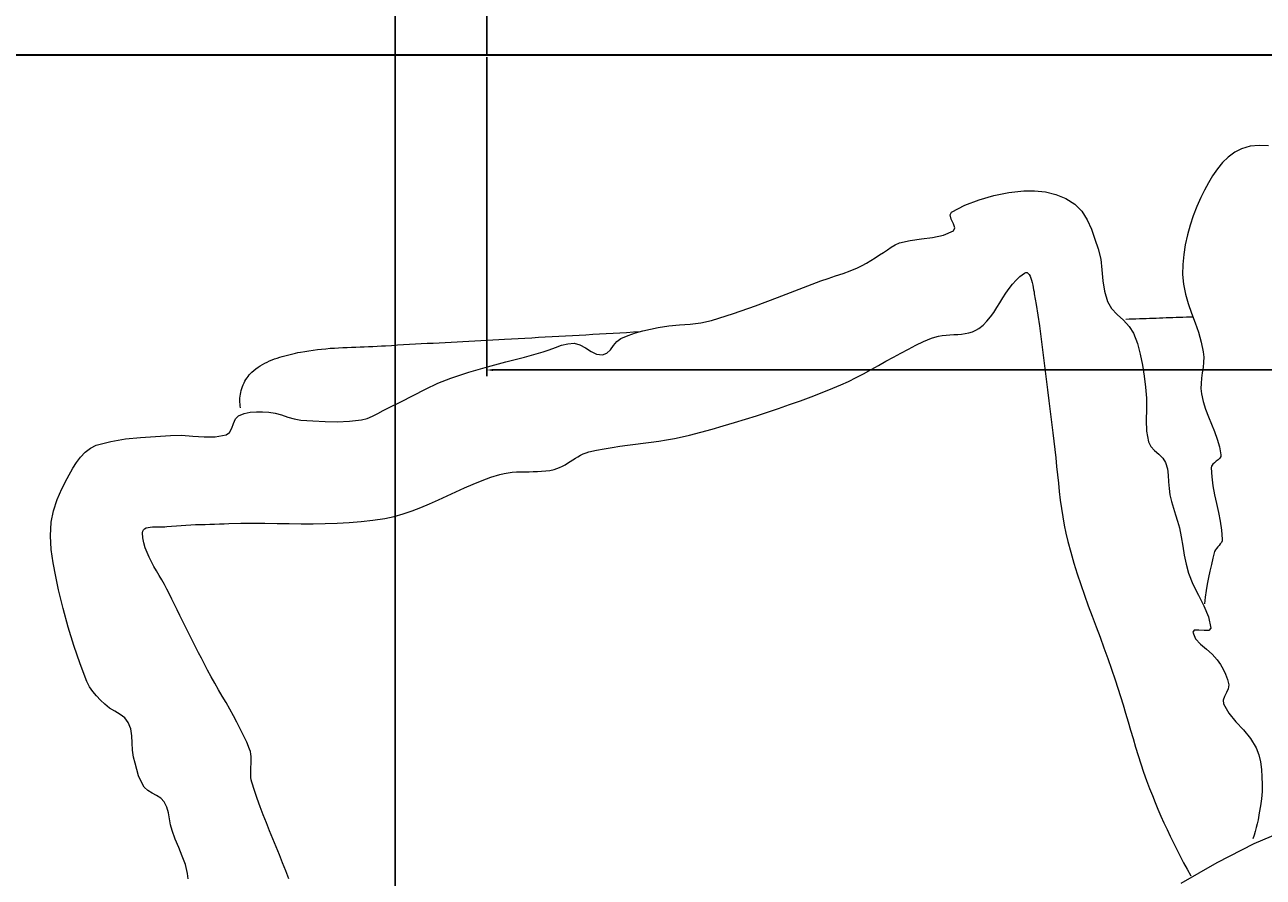
# Model space of a CAD drawing. Units: inches. Extents: x 1770 to 2988, y 1161 to 3221.
# Tile 16 of 44: x 2194 to 2229, y 2344 to 2369. Entities that reach past the tile are written whole.
import ezdxf

# ---------------------------------------------------------------- set-up
doc = ezdxf.new("R2010")
doc.units = ezdxf.units.IN
for name, color, linetype, lineweight in [('A-ANNO-DIMS', 2, 'Continuous', 18), ('A-FURN', 8, 'Continuous', 13), ('A-GLAZ', 4, 'Continuous', 18), ('A-WALL', 7, 'Continuous', 35)]:
    doc.layers.add(name, color=color, linetype=linetype, lineweight=lineweight)
doc.styles.get("Standard").update_dxf_attribs({"font": 'arial.ttf'})
doc.dimstyles.get("Standard").update_dxf_attribs({"dimtxt": 0.18, "dimasz": 0.18, "dimexe": 0.18, "dimexo": 0.0625, "dimgap": 0.09, "dimtad": 0, "dimtih": 1, "dimtoh": 1, "dimdec": 4, "dimzin": 0, "dimdsep": 46, "dimtxsty": 'Standard', "dimcen": 0.09, "dimadec": 0, "dimazin": 0, "dimtfac": 1, "dimtdec": 4, "dimtofl": 0, "dimtmove": 0, "dimatfit": 3, "dimfxl": 1, "dimtolj": 1, "dimtzin": 0, "dimarcsym": 0})

# ---------------------------------------------------------------- blocks, each defined once
blk = doc.blocks.new('BED-DOUBLE-PLAN')
for p, q in [((35.385, 105.421), (35.203, 105.287)), ((35.584, 105.525), (35.385, 105.421)), ((35.831, 105.596), (35.584, 105.525)), ((36.086, 105.618), (35.831, 105.596)), ((36.348, 105.604), (36.086, 105.618)), ((35.039, 105.128), (34.89, 104.949)), ((35.203, 105.287), (35.039, 105.128)), ((34.755, 104.754), (34.633, 104.551)), ((34.89, 104.949), (34.755, 104.754)), ((34.633, 104.551), (34.523, 104.343)), ((27.681, 103.909), (28.087, 104.068)), ((28.087, 104.068), (28.506, 104.19)), ((28.506, 104.19), (28.933, 104.274)), ((28.933, 104.274), (29.364, 104.322)), ((29.364, 104.322), (29.669, 104.325)), ((29.669, 104.325), (29.977, 104.292)), ((29.977, 104.292), (30.279, 104.22)), ((30.279, 104.22), (30.562, 104.105)), ((30.562, 104.105), (30.817, 103.944)), ((34.422, 104.135), (34.307, 103.876)), ((34.523, 104.343), (34.422, 104.135)), ((27.256, 103.634), (27.295, 103.714)), ((27.295, 103.714), (27.681, 103.909)), ((30.817, 103.944), (31.018, 103.741)), ((31.018, 103.741), (31.173, 103.496)), ((34.307, 103.876), (34.203, 103.61)), ((27.291, 103.514), (27.256, 103.634)), ((27.352, 103.382), (27.291, 103.514)), ((27.388, 103.262), (27.352, 103.382)), ((31.173, 103.496), (31.294, 103.225)), ((34.112, 103.338), (34.035, 103.063)), ((34.203, 103.61), (34.112, 103.338)), ((26.119, 102.906), (26.438, 102.948)), ((26.438, 102.948), (26.756, 102.988)), ((26.756, 102.988), (27.064, 103.056)), ((27.064, 103.056), (27.349, 103.179)), ((27.349, 103.179), (27.388, 103.262)), ((31.294, 103.225), (31.395, 102.942)), ((31.395, 102.942), (31.487, 102.661)), ((34.035, 103.063), (33.974, 102.783)), ((25.354, 102.561), (25.464, 102.639)), ((25.464, 102.639), (25.574, 102.714)), ((25.574, 102.714), (25.689, 102.781)), ((25.689, 102.781), (25.811, 102.832)), ((25.811, 102.832), (26.119, 102.906)), ((31.487, 102.661), (31.558, 102.366)), ((33.974, 102.783), (33.93, 102.502)), ((24.742, 102.187), (24.869, 102.258)), ((24.869, 102.258), (24.993, 102.335)), ((24.993, 102.335), (25.117, 102.412)), ((25.117, 102.412), (25.242, 102.489)), ((25.242, 102.489), (25.354, 102.561)), ((31.558, 102.366), (31.593, 102.061)), ((33.93, 102.502), (33.904, 102.219)), ((23.778, 101.819), (23.988, 101.89)), ((23.988, 101.89), (24.198, 101.962)), ((24.198, 101.962), (24.406, 102.038)), ((24.406, 102.038), (24.611, 102.123)), ((24.611, 102.123), (24.742, 102.187)), ((29.139, 101.774), (29.253, 101.879)), ((29.253, 101.879), (29.38, 101.971)), ((29.38, 101.971), (29.42, 101.987)), ((29.42, 101.987), (29.457, 101.984)), ((29.457, 101.984), (29.489, 101.964)), ((29.489, 101.964), (29.518, 101.93)), ((29.518, 101.93), (29.543, 101.885)), ((29.543, 101.885), (29.566, 101.829)), ((31.593, 102.061), (31.62, 101.753)), ((33.904, 102.219), (33.898, 101.936)), ((33.898, 101.936), (33.922, 101.653)), ((22.945, 101.514), (23.568, 101.747)), ((23.568, 101.747), (23.778, 101.819)), ((28.85, 101.399), (28.939, 101.531)), ((28.939, 101.531), (29.035, 101.657)), ((29.035, 101.657), (29.139, 101.774)), ((29.566, 101.829), (29.586, 101.767)), ((29.586, 101.767), (29.603, 101.7)), ((29.603, 101.7), (29.618, 101.631)), ((29.618, 101.631), (29.631, 101.561)), ((29.631, 101.561), (29.643, 101.495)), ((31.62, 101.753), (31.664, 101.452)), ((33.922, 101.653), (33.978, 101.374)), ((21.701, 101.039), (22.324, 101.275)), ((22.324, 101.275), (22.945, 101.514)), ((28.679, 101.123), (28.763, 101.262)), ((28.763, 101.262), (28.85, 101.399)), ((29.643, 101.495), (29.653, 101.433)), ((29.653, 101.433), (29.662, 101.379)), ((29.662, 101.379), (29.714, 101.076)), ((31.664, 101.452), (31.751, 101.162)), ((33.978, 101.374), (34.058, 101.099)), ((20.44, 100.618), (21.074, 100.817)), ((21.074, 100.817), (21.701, 101.039)), ((28.411, 100.721), (28.505, 100.85)), ((28.505, 100.85), (28.593, 100.985)), ((28.593, 100.985), (28.679, 101.123)), ((29.714, 101.076), (29.763, 100.772)), ((31.751, 101.162), (31.871, 100.963)), ((31.871, 100.963), (32.032, 100.788)), ((34.058, 101.099), (34.153, 100.826)), ((34.153, 100.826), (34.252, 100.553)), ((18.918, 100.416), (19.222, 100.462)), ((19.222, 100.462), (19.529, 100.49)), ((19.529, 100.49), (19.836, 100.515)), ((19.836, 100.515), (20.141, 100.553)), ((20.141, 100.553), (20.44, 100.618)), ((28.077, 100.392), (28.2, 100.489)), ((28.2, 100.489), (28.31, 100.6)), ((28.31, 100.6), (28.411, 100.721)), ((29.763, 100.772), (29.808, 100.467)), ((29.808, 100.467), (29.85, 100.162)), ((32.032, 100.788), (32.208, 100.623)), ((32.208, 100.623), (32.371, 100.449)), ((32.279, 100.659), (32.375, 100.663)), ((32.375, 100.663), (32.47, 100.666)), ((32.47, 100.666), (32.566, 100.669)), ((32.566, 100.669), (32.662, 100.673)), ((32.662, 100.673), (32.758, 100.676)), ((32.758, 100.676), (32.854, 100.679)), ((32.854, 100.679), (32.949, 100.683)), ((32.949, 100.683), (33.045, 100.686)), ((33.045, 100.686), (33.141, 100.689)), ((33.141, 100.689), (33.237, 100.693)), ((33.237, 100.693), (33.333, 100.696)), ((33.333, 100.696), (33.429, 100.7)), ((33.429, 100.7), (33.524, 100.703)), ((33.524, 100.703), (33.62, 100.706)), ((33.62, 100.706), (33.716, 100.71)), ((33.716, 100.71), (33.812, 100.713)), ((33.812, 100.713), (33.908, 100.716)), ((33.908, 100.716), (34.004, 100.72)), ((34.004, 100.72), (34.099, 100.723)), ((34.099, 100.723), (34.195, 100.726)), ((34.252, 100.553), (34.347, 100.28)), ((14.92, 100.104), (15.114, 100.115)), ((15.114, 100.115), (15.308, 100.126)), ((15.308, 100.126), (15.501, 100.137)), ((15.501, 100.137), (15.695, 100.147)), ((15.695, 100.147), (15.888, 100.158)), ((15.888, 100.158), (16.082, 100.169)), ((16.082, 100.169), (16.276, 100.18)), ((16.276, 100.18), (16.469, 100.191)), ((16.469, 100.191), (16.663, 100.202)), ((16.663, 100.202), (16.857, 100.213)), ((16.857, 100.213), (17.05, 100.224)), ((17.05, 100.224), (17.244, 100.235)), ((17.244, 100.235), (17.437, 100.246)), ((17.437, 100.246), (17.631, 100.257)), ((17.631, 100.257), (17.825, 100.268)), ((17.825, 100.268), (18.018, 100.279)), ((17.853, 100.102), (18.057, 100.19)), ((18.018, 100.279), (18.212, 100.29)), ((18.057, 100.19), (18.267, 100.262)), ((18.212, 100.29), (18.406, 100.301)), ((18.267, 100.262), (18.482, 100.321)), ((18.482, 100.321), (18.7, 100.371)), ((18.7, 100.371), (18.918, 100.416)), ((26.5, 100.015), (26.723, 100.111)), ((26.723, 100.111), (26.823, 100.146)), ((26.823, 100.146), (26.927, 100.171)), ((26.927, 100.171), (27.034, 100.188)), ((27.034, 100.188), (27.143, 100.2)), ((27.143, 100.2), (27.253, 100.208)), ((27.253, 100.208), (27.363, 100.215)), ((27.363, 100.215), (27.473, 100.222)), ((27.473, 100.222), (27.582, 100.232)), ((27.582, 100.232), (27.688, 100.246)), ((27.688, 100.246), (27.792, 100.267)), ((27.792, 100.267), (27.892, 100.297)), ((27.892, 100.297), (27.987, 100.338)), ((27.987, 100.338), (28.077, 100.392)), ((29.85, 100.162), (29.89, 99.857)), ((32.371, 100.449), (32.495, 100.252)), ((32.495, 100.252), (32.606, 99.957)), ((34.347, 100.28), (34.429, 100.003)), ((8.824, 99.736), (8.944, 99.756)), ((8.944, 99.756), (9.065, 99.773)), ((9.065, 99.773), (9.185, 99.788)), ((9.185, 99.788), (9.306, 99.802)), ((9.306, 99.802), (9.428, 99.813)), ((9.428, 99.813), (9.549, 99.823)), ((9.549, 99.823), (9.671, 99.831)), ((9.671, 99.831), (9.792, 99.839)), ((9.792, 99.839), (9.914, 99.845)), ((9.914, 99.845), (10.036, 99.851)), ((10.036, 99.851), (10.158, 99.855)), ((10.158, 99.855), (10.28, 99.86)), ((10.28, 99.86), (10.403, 99.864)), ((10.403, 99.864), (10.525, 99.869)), ((10.525, 99.869), (10.647, 99.873)), ((10.647, 99.873), (10.769, 99.878)), ((10.769, 99.878), (10.891, 99.883)), ((10.891, 99.883), (11.012, 99.89)), ((11.012, 99.89), (11.134, 99.897)), ((11.134, 99.897), (11.304, 99.907)), ((11.304, 99.907), (11.474, 99.918)), ((11.474, 99.918), (11.644, 99.928)), ((11.644, 99.928), (11.814, 99.938)), ((11.814, 99.938), (11.984, 99.947)), ((11.984, 99.947), (12.154, 99.957)), ((12.154, 99.957), (12.324, 99.966)), ((12.324, 99.966), (12.493, 99.975)), ((12.493, 99.975), (12.663, 99.984)), ((12.663, 99.984), (12.833, 99.993)), ((12.833, 99.993), (13.003, 100.002)), ((13.003, 100.002), (13.173, 100.011)), ((13.173, 100.011), (13.343, 100.019)), ((13.343, 100.019), (13.513, 100.028)), ((13.513, 100.028), (13.683, 100.037)), ((13.683, 100.037), (13.853, 100.046)), ((13.853, 100.046), (14.023, 100.055)), ((14.023, 100.055), (14.193, 100.064)), ((14.193, 100.064), (14.363, 100.073)), ((14.363, 100.073), (14.533, 100.083)), ((14.533, 100.083), (14.727, 100.093)), ((14.727, 100.093), (14.92, 100.104)), ((15.635, 99.718), (15.81, 99.777)), ((15.81, 99.777), (15.984, 99.845)), ((15.984, 99.845), (16.159, 99.909)), ((16.159, 99.909), (16.336, 99.954)), ((16.336, 99.954), (16.516, 99.966)), ((16.516, 99.966), (16.685, 99.923)), ((16.685, 99.923), (16.844, 99.835)), ((16.844, 99.835), (17.001, 99.735)), ((17.452, 99.683), (17.553, 99.78)), ((17.553, 99.78), (17.645, 99.9)), ((17.645, 99.9), (17.741, 100.016)), ((17.741, 100.016), (17.853, 100.102)), ((25.85, 99.689), (26.064, 99.803)), ((26.064, 99.803), (26.281, 99.912)), ((26.281, 99.912), (26.5, 100.015)), ((29.89, 99.857), (29.929, 99.551)), ((32.606, 99.957), (32.689, 99.653)), ((34.429, 100.003), (34.488, 99.723)), ((7.619, 99.363), (7.685, 99.399)), ((7.685, 99.399), (7.753, 99.432)), ((7.753, 99.432), (7.822, 99.463)), ((7.822, 99.463), (7.892, 99.493)), ((7.892, 99.493), (7.964, 99.52)), ((7.964, 99.52), (8.036, 99.546)), ((8.036, 99.546), (8.109, 99.569)), ((8.109, 99.569), (8.183, 99.591)), ((8.183, 99.591), (8.258, 99.612)), ((8.258, 99.612), (8.332, 99.632)), ((8.332, 99.632), (8.407, 99.65)), ((8.407, 99.65), (8.482, 99.667)), ((8.482, 99.667), (8.556, 99.684)), ((8.556, 99.684), (8.631, 99.699)), ((8.631, 99.699), (8.705, 99.714)), ((8.705, 99.714), (8.824, 99.736)), ((14.041, 99.297), (14.572, 99.437)), ((14.572, 99.437), (15.105, 99.574)), ((15.105, 99.574), (15.635, 99.718)), ((17.001, 99.735), (17.16, 99.657)), ((17.16, 99.657), (17.329, 99.635)), ((17.329, 99.635), (17.452, 99.683)), ((25.212, 99.334), (25.424, 99.453)), ((25.424, 99.453), (25.636, 99.572)), ((25.636, 99.572), (25.85, 99.689)), ((29.929, 99.551), (29.966, 99.246)), ((32.689, 99.653), (32.75, 99.342)), ((34.496, 99.425), (34.48, 99.274)), ((34.488, 99.723), (34.501, 99.574)), ((34.501, 99.574), (34.496, 99.425)), ((7.207, 99.023), (7.241, 99.066)), ((7.241, 99.066), (7.278, 99.106)), ((7.278, 99.106), (7.316, 99.144)), ((7.316, 99.144), (7.372, 99.193)), ((7.372, 99.193), (7.431, 99.24)), ((7.431, 99.24), (7.491, 99.283)), ((7.491, 99.283), (7.554, 99.324)), ((7.554, 99.324), (7.619, 99.363)), ((12.992, 98.973), (13.513, 99.145)), ((13.513, 99.145), (14.041, 99.297)), ((24.571, 98.986), (24.786, 99.099)), ((24.786, 99.099), (25, 99.215)), ((25, 99.215), (25.212, 99.334)), ((29.966, 99.246), (30.003, 98.94)), ((32.75, 99.342), (32.799, 99.027)), ((34.459, 99.124), (34.438, 98.973)), ((34.48, 99.274), (34.459, 99.124)), ((7.028, 98.674), (7.046, 98.728)), ((7.046, 98.728), (7.067, 98.781)), ((7.067, 98.781), (7.091, 98.833)), ((7.091, 98.833), (7.117, 98.883)), ((7.117, 98.883), (7.144, 98.931)), ((7.144, 98.931), (7.175, 98.978)), ((7.175, 98.978), (7.207, 99.023)), ((12.273, 98.658), (12.628, 98.826)), ((12.628, 98.826), (12.992, 98.973)), ((23.911, 98.681), (24.134, 98.776)), ((24.134, 98.776), (24.354, 98.878)), ((24.354, 98.878), (24.571, 98.986)), ((30.003, 98.94), (30.039, 98.634)), ((32.799, 99.027), (32.842, 98.713)), ((32.842, 98.713), (32.864, 98.4)), ((34.423, 98.823), (34.42, 98.674)), ((34.438, 98.973), (34.423, 98.823)), ((6.971, 98.342), (6.974, 98.397)), ((6.971, 98.287), (6.971, 98.342)), ((6.974, 98.397), (6.979, 98.453)), ((6.979, 98.453), (6.987, 98.509)), ((6.987, 98.509), (6.998, 98.565)), ((6.998, 98.565), (7.012, 98.62)), ((7.012, 98.62), (7.028, 98.674)), ((11.572, 98.299), (11.922, 98.48)), ((11.922, 98.48), (12.273, 98.658)), ((22.983, 98.327), (23.293, 98.442)), ((23.293, 98.442), (23.603, 98.56)), ((23.603, 98.56), (23.911, 98.681)), ((30.039, 98.634), (30.076, 98.328)), ((32.864, 98.4), (32.862, 98.084)), ((34.42, 98.674), (34.435, 98.525)), ((34.435, 98.525), (34.485, 98.303)), ((6.975, 98.232), (6.971, 98.287)), ((6.981, 98.178), (6.975, 98.232)), ((6.99, 98.125), (6.981, 98.178)), ((7.094, 97.962), (7.265, 97.998)), ((7.265, 97.998), (7.442, 98.012)), ((7.442, 98.012), (7.621, 98.01)), ((7.621, 98.01), (7.798, 98)), ((7.798, 98), (7.983, 97.971)), ((10.916, 97.961), (11.066, 98.046)), ((11.066, 98.046), (11.219, 98.125)), ((11.219, 98.125), (11.572, 98.299)), ((21.728, 97.898), (22.043, 98)), ((22.043, 98), (22.358, 98.106)), ((22.358, 98.106), (22.671, 98.215)), ((22.671, 98.215), (22.983, 98.327)), ((30.076, 98.328), (30.113, 98.022)), ((30.113, 98.022), (30.152, 97.716)), ((32.862, 98.084), (32.856, 97.768)), ((34.485, 98.303), (34.554, 98.085)), ((34.554, 98.085), (34.635, 97.87)), ((6.737, 97.54), (6.785, 97.678)), ((6.785, 97.678), (6.843, 97.807)), ((6.843, 97.807), (6.934, 97.897)), ((6.934, 97.897), (7.094, 97.962)), ((7.983, 97.971), (8.164, 97.919)), ((8.164, 97.919), (8.344, 97.86)), ((8.344, 97.86), (8.526, 97.807)), ((8.526, 97.807), (8.711, 97.775)), ((8.711, 97.775), (9.057, 97.749)), ((9.057, 97.749), (9.404, 97.731)), ((9.404, 97.731), (9.752, 97.727)), ((9.752, 97.727), (10.099, 97.741)), ((10.099, 97.741), (10.443, 97.776)), ((10.443, 97.776), (10.607, 97.816)), ((10.607, 97.816), (10.764, 97.881)), ((10.764, 97.881), (10.916, 97.961)), ((20.777, 97.608), (21.095, 97.702)), ((21.095, 97.702), (21.412, 97.798)), ((21.412, 97.798), (21.728, 97.898)), ((30.152, 97.716), (30.192, 97.411)), ((32.856, 97.768), (32.868, 97.455)), ((34.635, 97.87), (34.722, 97.657)), ((34.722, 97.657), (34.808, 97.443)), ((3.703, 97.235), (4.13, 97.276)), ((4.13, 97.276), (4.56, 97.305)), ((4.56, 97.305), (4.988, 97.334)), ((4.988, 97.334), (5.307, 97.338)), ((5.307, 97.338), (5.628, 97.316)), ((5.628, 97.316), (5.949, 97.294)), ((5.949, 97.294), (6.266, 97.297)), ((6.266, 97.297), (6.576, 97.352)), ((6.576, 97.352), (6.675, 97.422)), ((6.675, 97.422), (6.737, 97.54)), ((19.381, 97.247), (19.6, 97.292)), ((19.6, 97.292), (19.818, 97.344)), ((19.818, 97.344), (20.138, 97.429)), ((20.138, 97.429), (20.458, 97.517)), ((20.458, 97.517), (20.777, 97.608)), ((30.192, 97.411), (30.222, 97.172)), ((32.868, 97.455), (32.921, 97.148)), ((34.808, 97.443), (34.886, 97.228)), ((2.554, 96.859), (2.703, 96.975)), ((2.703, 96.975), (2.87, 97.055)), ((2.87, 97.055), (3.281, 97.166)), ((3.281, 97.166), (3.703, 97.235)), ((17.161, 96.913), (17.38, 96.957)), ((17.38, 96.957), (17.602, 96.995)), ((17.602, 96.995), (17.824, 97.028)), ((17.824, 97.028), (18.046, 97.058)), ((18.046, 97.058), (18.269, 97.086)), ((18.269, 97.086), (18.493, 97.114)), ((18.493, 97.114), (18.716, 97.143)), ((18.716, 97.143), (18.938, 97.174)), ((18.938, 97.174), (19.16, 97.208)), ((19.16, 97.208), (19.381, 97.247)), ((30.222, 97.172), (30.25, 96.932)), ((30.25, 96.932), (30.275, 96.692)), ((32.921, 97.148), (32.988, 97.015)), ((32.988, 97.015), (33.094, 96.903)), ((34.886, 97.228), (34.95, 97.009)), ((34.95, 97.009), (34.993, 96.785)), ((2.307, 96.562), (2.422, 96.718)), ((2.422, 96.718), (2.554, 96.859)), ((16.332, 96.542), (16.406, 96.589)), ((16.406, 96.589), (16.48, 96.636)), ((16.48, 96.636), (16.554, 96.682)), ((16.554, 96.682), (16.628, 96.726)), ((16.628, 96.726), (16.704, 96.768)), ((16.704, 96.768), (16.781, 96.805)), ((16.781, 96.805), (16.86, 96.837)), ((16.86, 96.837), (16.942, 96.862)), ((16.942, 96.862), (17.161, 96.913)), ((30.275, 96.692), (30.3, 96.452)), ((33.094, 96.903), (33.215, 96.799)), ((33.215, 96.799), (33.328, 96.689)), ((33.328, 96.689), (33.41, 96.561)), ((34.86, 96.597), (34.806, 96.555)), ((34.912, 96.639), (34.86, 96.597)), ((34.957, 96.683), (34.912, 96.639)), ((34.986, 96.731), (34.957, 96.683)), ((34.993, 96.785), (34.986, 96.731)), ((2.039, 96.109), (2.205, 96.4)), ((2.205, 96.4), (2.307, 96.562)), ((14.142, 96.14), (14.4, 96.222)), ((14.4, 96.222), (14.516, 96.251)), ((14.516, 96.251), (14.632, 96.271)), ((14.632, 96.271), (14.751, 96.284)), ((14.751, 96.284), (14.87, 96.293)), ((14.87, 96.293), (14.99, 96.297)), ((14.99, 96.297), (15.11, 96.299)), ((15.11, 96.299), (15.23, 96.299)), ((15.23, 96.299), (15.351, 96.301)), ((15.351, 96.301), (15.471, 96.304)), ((15.471, 96.304), (15.591, 96.31)), ((15.591, 96.31), (15.71, 96.321)), ((15.71, 96.321), (15.827, 96.338)), ((15.827, 96.338), (15.944, 96.363)), ((15.944, 96.363), (16.026, 96.388)), ((16.026, 96.388), (16.105, 96.419)), ((16.105, 96.419), (16.182, 96.456)), ((16.182, 96.456), (16.258, 96.498)), ((16.258, 96.498), (16.332, 96.542)), ((30.3, 96.452), (30.324, 96.211)), ((33.41, 96.561), (33.462, 96.384)), ((33.462, 96.384), (33.486, 96.199)), ((34.725, 96.462), (34.713, 96.407)), ((34.713, 96.407), (34.729, 96.151)), ((34.759, 96.511), (34.725, 96.462)), ((34.806, 96.555), (34.759, 96.511)), ((1.884, 95.809), (2.039, 96.109)), ((13.385, 95.836), (13.635, 95.945)), ((13.635, 95.945), (13.887, 96.047)), ((13.887, 96.047), (14.142, 96.14)), ((30.324, 96.211), (30.349, 95.971)), ((30.349, 95.971), (30.375, 95.731)), ((33.486, 96.199), (33.497, 96.01)), ((33.497, 96.01), (33.509, 95.822)), ((34.729, 96.151), (34.763, 95.896)), ((34.763, 95.896), (34.811, 95.643)), ((1.749, 95.501), (1.884, 95.809)), ((12.641, 95.494), (12.889, 95.608)), ((12.889, 95.608), (13.137, 95.723)), ((13.137, 95.723), (13.385, 95.836)), ((30.375, 95.731), (30.404, 95.491)), ((33.509, 95.822), (33.535, 95.636)), ((33.535, 95.636), (33.582, 95.446)), ((34.811, 95.643), (34.865, 95.39)), ((1.583, 94.858), (1.646, 95.184)), ((1.646, 95.184), (1.749, 95.501)), ((11.633, 95.096), (11.889, 95.182)), ((11.889, 95.182), (12.142, 95.279)), ((12.142, 95.279), (12.392, 95.383)), ((12.392, 95.383), (12.641, 95.494)), ((30.404, 95.491), (30.436, 95.252)), ((30.436, 95.252), (30.473, 95.014)), ((33.582, 95.446), (33.638, 95.258)), ((33.638, 95.258), (33.698, 95.071)), ((34.865, 95.39), (34.921, 95.137)), ((1.562, 94.471), (1.583, 94.858)), ((5.976, 94.796), (6.112, 94.8)), ((6.112, 94.8), (6.249, 94.804)), ((6.249, 94.804), (6.385, 94.808)), ((6.385, 94.808), (6.522, 94.812)), ((6.522, 94.812), (6.658, 94.817)), ((6.658, 94.817), (7.001, 94.826)), ((7.001, 94.826), (7.344, 94.829)), ((7.344, 94.829), (7.688, 94.827)), ((7.688, 94.827), (8.032, 94.823)), ((8.032, 94.823), (8.376, 94.818)), ((8.376, 94.818), (8.721, 94.814)), ((8.721, 94.814), (9.064, 94.813)), ((9.064, 94.813), (9.408, 94.816)), ((9.408, 94.816), (9.75, 94.826)), ((9.75, 94.826), (10.092, 94.844)), ((10.092, 94.844), (10.433, 94.873)), ((10.433, 94.873), (10.772, 94.913)), ((10.772, 94.913), (11.11, 94.966)), ((11.11, 94.966), (11.374, 95.023)), ((11.374, 95.023), (11.633, 95.096)), ((30.473, 95.014), (30.515, 94.777)), ((33.698, 95.071), (33.755, 94.883)), ((33.755, 94.883), (33.806, 94.694)), ((34.921, 95.137), (34.971, 94.884)), ((34.971, 94.884), (35.009, 94.629)), ((1.584, 94.082), (1.562, 94.471)), ((4.189, 94.55), (4.196, 94.6)), ((4.202, 94.406), (4.189, 94.55)), ((4.196, 94.6), (4.217, 94.64)), ((4.217, 94.64), (4.251, 94.67)), ((4.251, 94.67), (4.296, 94.693)), ((4.296, 94.693), (4.35, 94.708)), ((4.35, 94.708), (4.412, 94.718)), ((4.412, 94.718), (4.479, 94.724)), ((4.479, 94.724), (4.55, 94.727)), ((4.55, 94.727), (4.622, 94.727)), ((4.622, 94.727), (4.693, 94.727)), ((4.693, 94.727), (4.762, 94.727)), ((4.762, 94.727), (4.827, 94.728)), ((4.827, 94.728), (4.886, 94.732)), ((4.886, 94.732), (5.022, 94.746)), ((5.022, 94.746), (5.158, 94.757)), ((5.158, 94.757), (5.294, 94.767)), ((5.294, 94.767), (5.43, 94.775)), ((5.43, 94.775), (5.566, 94.782)), ((5.566, 94.782), (5.703, 94.787)), ((5.703, 94.787), (5.839, 94.792)), ((5.839, 94.792), (5.976, 94.796)), ((30.515, 94.777), (30.563, 94.541)), ((30.563, 94.541), (30.618, 94.307)), ((33.806, 94.694), (33.859, 94.435)), ((35.009, 94.629), (35.031, 94.373)), ((4.229, 94.265), (4.202, 94.406)), ((4.269, 94.127), (4.229, 94.265)), ((4.319, 93.992), (4.269, 94.127)), ((30.618, 94.307), (30.701, 93.997)), ((33.859, 94.435), (33.903, 94.175)), ((33.903, 94.175), (33.946, 93.914)), ((34.863, 94.11), (34.833, 94.065)), ((34.899, 94.152), (34.863, 94.11)), ((34.938, 94.193), (34.899, 94.152)), ((34.974, 94.235), (34.938, 94.193)), ((35.004, 94.278), (34.974, 94.235)), ((35.024, 94.323), (35.004, 94.278)), ((35.031, 94.373), (35.024, 94.323)), ((1.637, 93.693), (1.584, 94.082)), ((4.378, 93.858), (4.319, 93.992)), ((4.444, 93.726), (4.378, 93.858)), ((30.701, 93.997), (30.791, 93.689)), ((33.946, 93.914), (33.997, 93.655)), ((34.763, 93.833), (34.718, 93.649)), ((34.812, 94.017), (34.763, 93.833)), ((34.833, 94.065), (34.812, 94.017)), ((1.711, 93.307), (1.637, 93.693)), ((4.515, 93.595), (4.444, 93.726)), ((4.59, 93.465), (4.515, 93.595)), ((4.666, 93.336), (4.59, 93.465)), ((30.791, 93.689), (30.887, 93.383)), ((33.997, 93.655), (34.064, 93.401)), ((34.064, 93.401), (34.191, 93.084)), ((34.676, 93.463), (34.637, 93.277)), ((34.718, 93.649), (34.676, 93.463)), ((1.795, 92.924), (1.711, 93.307)), ((4.742, 93.207), (4.666, 93.336)), ((4.817, 93.077), (4.742, 93.207)), ((4.888, 92.947), (4.817, 93.077)), ((30.887, 93.383), (30.989, 93.078)), ((30.989, 93.078), (31.095, 92.775)), ((34.191, 93.084), (34.349, 92.776)), ((34.602, 93.089), (34.571, 92.902)), ((34.637, 93.277), (34.602, 93.089)), ((1.923, 92.391), (1.795, 92.924)), ((4.953, 92.816), (4.888, 92.947)), ((5.027, 92.661), (4.953, 92.816)), ((31.095, 92.775), (31.204, 92.473)), ((34.349, 92.776), (34.507, 92.47)), ((34.543, 92.713), (34.519, 92.525)), ((34.571, 92.902), (34.543, 92.713)), ((2.067, 91.861), (1.923, 92.391)), ((5.102, 92.506), (5.027, 92.661)), ((5.177, 92.351), (5.102, 92.506)), ((5.252, 92.197), (5.177, 92.351)), ((31.204, 92.473), (31.315, 92.172)), ((34.507, 92.47), (34.635, 92.156)), ((5.328, 92.043), (5.252, 92.197)), ((5.405, 91.889), (5.328, 92.043)), ((31.315, 92.172), (31.427, 91.87)), ((34.635, 92.156), (34.701, 91.828)), ((2.227, 91.336), (2.067, 91.861)), ((5.482, 91.736), (5.405, 91.889)), ((5.559, 91.583), (5.482, 91.736)), ((31.427, 91.87), (31.54, 91.569)), ((34.229, 91.774), (34.188, 91.712)), ((34.188, 91.712), (34.269, 91.526)), ((34.357, 91.777), (34.229, 91.774)), ((34.516, 91.761), (34.357, 91.777)), ((34.649, 91.765), (34.516, 91.761)), ((34.701, 91.828), (34.649, 91.765)), ((2.405, 90.816), (2.227, 91.336)), ((5.637, 91.43), (5.559, 91.583)), ((5.715, 91.277), (5.637, 91.43)), ((5.794, 91.124), (5.715, 91.277)), ((31.54, 91.569), (31.652, 91.268)), ((31.652, 91.268), (31.762, 90.966)), ((34.269, 91.526), (34.408, 91.37)), ((34.408, 91.37), (34.576, 91.228)), ((5.872, 90.971), (5.794, 91.124)), ((5.951, 90.819), (5.872, 90.971)), ((31.762, 90.966), (31.869, 90.663)), ((34.576, 91.228), (34.746, 91.085)), ((34.746, 91.085), (34.888, 90.925)), ((34.888, 90.925), (34.975, 90.793)), ((2.601, 90.304), (2.405, 90.816)), ((6.05, 90.63), (5.951, 90.819)), ((6.153, 90.443), (6.05, 90.63)), ((31.869, 90.663), (31.973, 90.359)), ((34.975, 90.793), (35.056, 90.655)), ((35.056, 90.655), (35.126, 90.512)), ((2.675, 90.157), (2.601, 90.304)), ((6.258, 90.258), (6.153, 90.443)), ((6.364, 90.073), (6.258, 90.258)), ((31.973, 90.359), (32.05, 90.12)), ((35.126, 90.512), (35.181, 90.364)), ((35.181, 90.364), (35.215, 90.211)), ((35.215, 90.211), (35.201, 90.1)), ((2.769, 90.021), (2.675, 90.157)), ((2.877, 89.894), (2.769, 90.021)), ((2.994, 89.773), (2.877, 89.894)), ((6.47, 89.888), (6.364, 90.073)), ((6.577, 89.703), (6.47, 89.888)), ((32.05, 90.12), (32.125, 89.88)), ((32.125, 89.88), (32.197, 89.64)), ((35.091, 89.882), (35.052, 89.775)), ((35.151, 89.99), (35.091, 89.882)), ((35.201, 90.1), (35.151, 89.99)), ((3.112, 89.656), (2.994, 89.773)), ((3.247, 89.55), (3.112, 89.656)), ((3.397, 89.459), (3.247, 89.55)), ((6.682, 89.518), (6.577, 89.703)), ((6.786, 89.331), (6.682, 89.518)), ((32.197, 89.64), (32.269, 89.399)), ((35.052, 89.775), (35.063, 89.671)), ((35.063, 89.671), (35.219, 89.402)), ((3.548, 89.369), (3.397, 89.459)), ((3.682, 89.267), (3.548, 89.369)), ((3.785, 89.136), (3.682, 89.267)), ((6.886, 89.144), (6.786, 89.331)), ((6.984, 88.955), (6.886, 89.144)), ((32.269, 89.399), (32.34, 89.158)), ((32.34, 89.158), (32.41, 88.917)), ((35.219, 89.402), (35.418, 89.158)), ((35.418, 89.158), (35.633, 88.923)), ((3.854, 88.952), (3.785, 89.136)), ((3.883, 88.756), (3.854, 88.952)), ((7.077, 88.764), (6.984, 88.955)), ((32.41, 88.917), (32.481, 88.676)), ((35.633, 88.923), (35.836, 88.68)), ((3.892, 88.552), (3.883, 88.756)), ((3.902, 88.348), (3.892, 88.552)), ((7.166, 88.571), (7.077, 88.764)), ((7.248, 88.375), (7.166, 88.571)), ((32.481, 88.676), (32.554, 88.436)), ((32.554, 88.436), (32.628, 88.196)), ((35.836, 88.68), (36.001, 88.415)), ((3.933, 88.15), (3.902, 88.348)), ((3.976, 87.971), (3.933, 88.15)), ((7.271, 88.306), (7.248, 88.375)), ((7.286, 88.236), (7.271, 88.306)), ((7.294, 88.164), (7.286, 88.236)), ((7.296, 88.091), (7.294, 88.164)), ((7.295, 88.017), (7.296, 88.091)), ((32.628, 88.196), (32.705, 87.957)), ((36.001, 88.415), (36.077, 88.217)), ((36.077, 88.217), (36.124, 88.01)), ((4.024, 87.792), (3.976, 87.971)), ((4.08, 87.617), (4.024, 87.792)), ((7.28, 87.718), (7.283, 87.792)), ((7.283, 87.792), (7.287, 87.867)), ((7.287, 87.867), (7.292, 87.942)), ((7.292, 87.942), (7.295, 88.017)), ((32.705, 87.957), (32.785, 87.719)), ((36.124, 88.01), (36.151, 87.797)), ((36.151, 87.797), (36.164, 87.581)), ((4.151, 87.448), (4.08, 87.617)), ((4.242, 87.291), (4.151, 87.448)), ((7.28, 87.644), (7.28, 87.718)), ((7.285, 87.57), (7.28, 87.644)), ((7.295, 87.498), (7.285, 87.57)), ((7.312, 87.428), (7.295, 87.498)), ((7.387, 87.194), (7.312, 87.428)), ((32.785, 87.719), (32.868, 87.483)), ((32.868, 87.483), (32.956, 87.248)), ((36.164, 87.581), (36.171, 87.367)), ((4.34, 87.192), (4.242, 87.291)), ((4.463, 87.117), (4.34, 87.192)), ((4.593, 87.049), (4.463, 87.117)), ((4.715, 86.973), (4.593, 87.049)), ((7.467, 86.961), (7.387, 87.194)), ((32.956, 87.248), (33.033, 87.051)), ((33.033, 87.051), (33.113, 86.854)), ((36.167, 87.163), (36.149, 86.96)), ((36.171, 87.367), (36.167, 87.163)), ((4.809, 86.872), (4.715, 86.973)), ((4.883, 86.721), (4.809, 86.872)), ((4.93, 86.558), (4.883, 86.721)), ((7.551, 86.73), (7.467, 86.961)), ((7.639, 86.501), (7.551, 86.73)), ((33.113, 86.854), (33.194, 86.659)), ((36.121, 86.757), (36.087, 86.555)), ((36.149, 86.96), (36.121, 86.757)), ((4.962, 86.388), (4.93, 86.558)), ((4.993, 86.218), (4.962, 86.388)), ((7.729, 86.272), (7.639, 86.501)), ((33.194, 86.659), (33.278, 86.464)), ((33.278, 86.464), (33.364, 86.271)), ((36.051, 86.354), (36.029, 86.243)), ((36.087, 86.555), (36.051, 86.354)), ((5.036, 86.052), (4.993, 86.218)), ((5.126, 85.807), (5.036, 86.052)), ((7.821, 86.044), (7.729, 86.272)), ((7.914, 85.816), (7.821, 86.044)), ((33.364, 86.271), (33.453, 86.078)), ((33.453, 86.078), (33.543, 85.886)), ((37.023, 86.135), (35.936, 85.668)), ((35.973, 86.026), (35.938, 85.919)), ((36.003, 86.134), (35.973, 86.026)), ((36.029, 86.243), (36.003, 86.134)), ((5.227, 85.565), (5.126, 85.807)), ((8.007, 85.588), (7.914, 85.816)), ((33.543, 85.886), (33.636, 85.696)), ((33.636, 85.696), (33.73, 85.506)), ((35.936, 85.668), (34.877, 85.131)), ((35.938, 85.919), (35.899, 85.813)), ((5.327, 85.323), (5.227, 85.565)), ((5.414, 85.077), (5.327, 85.323)), ((8.101, 85.361), (8.007, 85.588)), ((8.193, 85.133), (8.101, 85.361)), ((33.73, 85.506), (33.827, 85.318)), ((33.827, 85.318), (33.926, 85.131)), ((5.478, 84.825), (5.414, 85.077)), ((8.284, 84.904), (8.193, 85.133)), ((8.372, 84.675), (8.284, 84.904)), ((34.877, 85.131), (33.846, 84.541)), ((33.926, 85.131), (34.027, 84.945)), ((34.027, 84.945), (34.13, 84.76)), ((5.49, 84.67), (5.478, 84.825))]:
    blk.add_line(p, q)
blk = doc.blocks.new('WIN-60-EXT')
for p, q in [((0, 9), (0, 0)), ((0, 0), (0, 4.5))]:
    blk.add_line(p, q)
blk = doc.blocks.new('*D30')
at = {"layer": 'A-ANNO-DIMS', "color": 0, "lineweight": -2, "transparency": 16777216}
for p, q in [((2207.278, 2367.64), (2207.278, 2358.522)), ((2267.278, 2367.64), (2267.278, 2358.522)), ((2207.458, 2358.702), (2235.853, 2358.702)), ((2267.098, 2358.702), (2238.702, 2358.702))]:
    blk.add_line(p, q, dxfattribs=at)
at = {"layer": 'A-ANNO-DIMS', "color": 0, "transparency": 16777216}
for points in [[(2207.458, 2358.732), (2207.458, 2358.672), (2207.278, 2358.702)], [(2267.098, 2358.732), (2267.098, 2358.672), (2267.278, 2358.702)]]:
    blk.add_solid(points, dxfattribs=at)
at = {"layer": 'Defpoints', "color": 0, "transparency": 16777216}
for p in [(2207.278, 2367.702), (2267.278, 2367.702), (2267.278, 2358.702)]:
    blk.add_point(p, dxfattribs=at)
at = {"layer": 'A-ANNO-DIMS', "color": 0, "transparency": 16777216, "insert": (2237.278, 2358.702), "char_height": 0.18, "attachment_point": 5}
blk.add_mtext('\\A1;EXT. WINDOW 60 TYP.', dxfattribs=at)
blk = doc.blocks.new('*D73')
at = {"layer": 'A-ANNO-DIMS', "color": 0, "lineweight": -2, "transparency": 16777216}
for p, q in [((2456.133, 2367.702), (1907.104, 2367.702)), ((1907.284, 2367.522), (1907.284, 2319.884)), ((1907.284, 2271.882), (1907.284, 2319.52)), ((2456.133, 2271.702), (1907.104, 2271.702))]:
    blk.add_line(p, q, dxfattribs=at)
at = {"layer": 'A-ANNO-DIMS', "color": 0, "transparency": 16777216}
for points in [[(1907.254, 2367.522), (1907.314, 2367.522), (1907.284, 2367.702)], [(1907.254, 2271.882), (1907.314, 2271.882), (1907.284, 2271.702)]]:
    blk.add_solid(points, dxfattribs=at)
at = {"layer": 'Defpoints', "color": 0, "transparency": 16777216}
for p in [(1907.284, 2367.702), (2456.196, 2367.702), (2456.196, 2271.702)]:
    blk.add_point(p, dxfattribs=at)
at = {"layer": 'A-ANNO-DIMS', "color": 0, "transparency": 16777216, "insert": (1907.284, 2319.702), "char_height": 0.18, "attachment_point": 5}
blk.add_mtext('\\A1;96', dxfattribs=at)
blk = doc.blocks.new('*D79')
at = {"layer": 'A-ANNO-DIMS', "color": 0, "lineweight": -2, "transparency": 16777216}
for p, q in [((2151.696, 1610.265), (2151.696, 2570.705)), ((2204.657, 1610.265), (2204.657, 2570.705)), ((2151.876, 2570.525), (2177.783, 2570.525)), ((2204.477, 2570.525), (2178.57, 2570.525))]:
    blk.add_line(p, q, dxfattribs=at)
at = {"layer": 'A-ANNO-DIMS', "color": 0, "transparency": 16777216}
for points in [[(2151.876, 2570.555), (2151.876, 2570.495), (2151.696, 2570.525)], [(2204.477, 2570.555), (2204.477, 2570.495), (2204.657, 2570.525)]]:
    blk.add_solid(points, dxfattribs=at)
at = {"layer": 'Defpoints', "color": 0, "transparency": 16777216}
for p in [(2204.657, 2570.525), (2151.696, 1610.202), (2204.657, 1610.202)]:
    blk.add_point(p, dxfattribs=at)
at = {"layer": 'A-ANNO-DIMS', "color": 0, "transparency": 16777216, "insert": (2178.176, 2570.525), "char_height": 0.18, "attachment_point": 5}
blk.add_mtext('\\A1;52.96', dxfattribs=at)

msp = doc.modelspace()

# ---------------------------------------------------------------- linework, layer by layer
at = {"layer": 'A-WALL'}
msp.add_line((2160.696, 2367.7021), (2328.696, 2367.7021), dxfattribs=at)

# ---------------------------------------------------------------- block references
at = {"layer": 'A-FURN'}
msp.add_blockref('BED-DOUBLE-PLAN', (2193.254, 2259.498), dxfattribs=at)
at = {"layer": 'A-GLAZ'}
msp.add_blockref('WIN-60-EXT', (2207.2778, 2367.702), dxfattribs=at)

# ---------------------------------------------------------------- dimensions: what is measured, and where the dimension line sits
at = {"layer": 'A-ANNO-DIMS'}
dim = msp.add_linear_dim(base=(2204.6568, 2570.5247), p1=(2151.696, 1610.2021), p2=(2204.6568, 1610.2021), dimstyle='Standard', override={"dimdec": 2, "dimlfac": 1, "dimrnd": 0, "dimzin": 0, "dimdsep": 46, "dimlunit": 2}, dxfattribs=at)
dim.commit()
dim.dimension.update_dxf_attribs({"geometry": '*D79', "text_midpoint": (2178.1764, 2570.5247)})
dim = msp.add_linear_dim(base=(1907.2844, 2367.7021), p1=(2456.196, 2271.7021), p2=(2456.196, 2367.7021), angle=90, dimstyle='Standard', override={"dimdec": 0, "dimlfac": 1, "dimrnd": 0, "dimzin": 0, "dimdsep": 46, "dimlunit": 2}, dxfattribs=at)
dim.commit()
dim.dimension.update_dxf_attribs({"geometry": '*D73', "text_midpoint": (1907.2844, 2319.7021)})
dim = msp.add_linear_dim(base=(2267.2776, 2358.7021), p1=(2207.2776, 2367.7021), p2=(2267.2776, 2367.7021), text='EXT. WINDOW <> TYP.', dimstyle='Standard', override={"dimdec": 0, "dimlfac": 1, "dimrnd": 0, "dimzin": 0, "dimdsep": 46, "dimlunit": 2}, dxfattribs=at)
dim.commit()
dim.dimension.update_dxf_attribs({"geometry": '*D30', "text_midpoint": (2237.2776, 2358.7021)})

doc.saveas('drawing.dxf')
